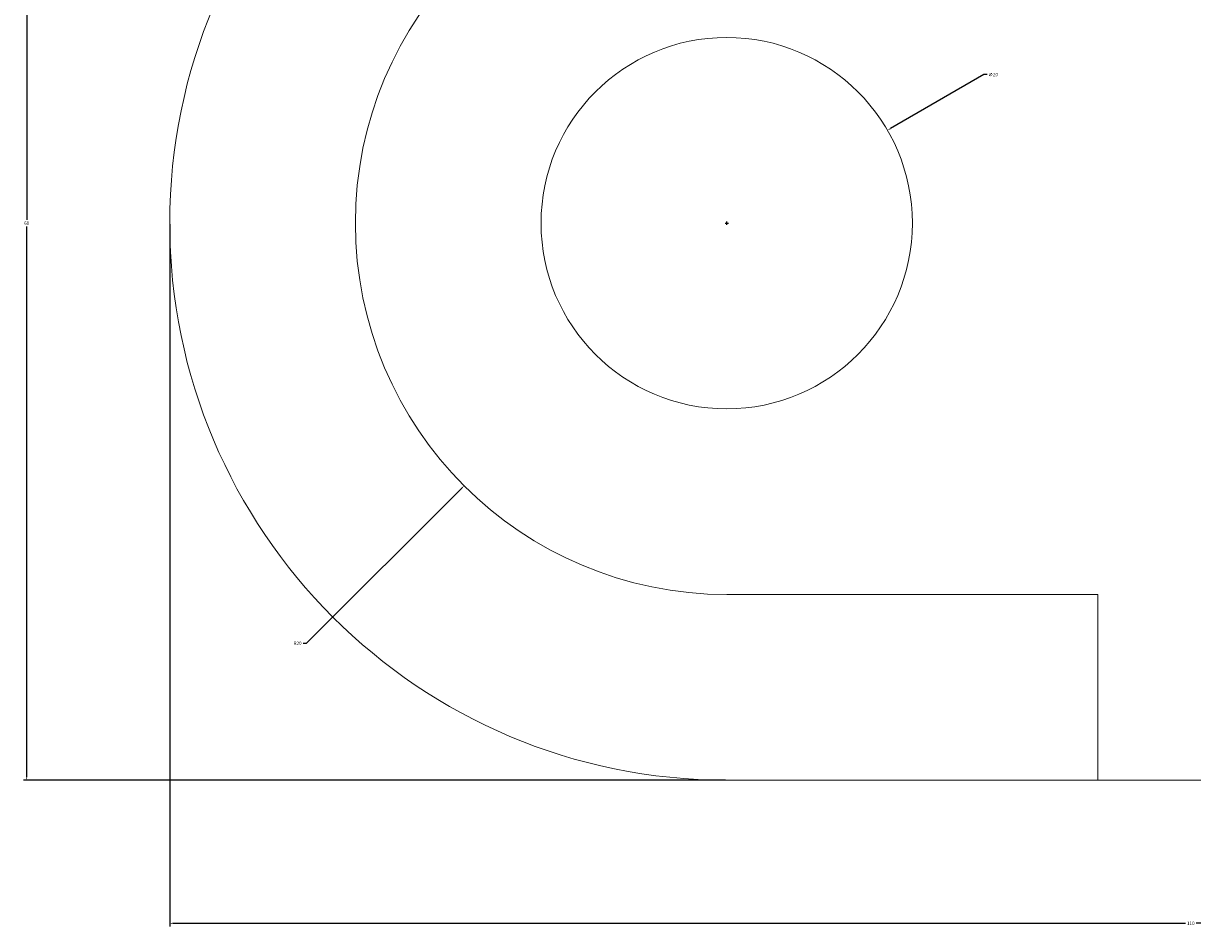
# Model space of a CAD drawing. Units: inches. Extents: x -19 to 107, y -27 to 49.
# Tile 1 of 4: x -19 to 44, y -27 to 22. Entities that reach past the tile are written whole.
import ezdxf

# ---------------------------------------------------------------- set-up
doc = ezdxf.new("R2010")
doc.units = ezdxf.units.IN
doc.header["$MEASUREMENT"] = 0
doc.layers.add('M-CONS', color=8, linetype='Continuous', lineweight=18)
doc.layers.add('M-DIMS', color=2, linetype='Continuous', lineweight=18)
doc.styles.get("Standard").update_dxf_attribs({"font": 'arial.ttf'})
doc.dimstyles.get("Standard").update_dxf_attribs({"dimtxt": 0.18, "dimasz": 0.18, "dimexe": 0.18, "dimexo": 0.0625, "dimgap": 0.09, "dimtad": 0, "dimtih": 1, "dimtoh": 1, "dimdec": 4, "dimzin": 0, "dimdsep": 46, "dimtxsty": 'Standard', "dimcen": 0.09, "dimadec": 0, "dimazin": 0, "dimtfac": 1, "dimtdec": 4, "dimtofl": 0, "dimtmove": 0, "dimatfit": 3, "dimfxl": 1, "dimtolj": 1, "dimtzin": 0, "dimarcsym": 0})

# ---------------------------------------------------------------- blocks, each defined once
blk = doc.blocks.new('*D1')
at = {"layer": 'Defpoints', "color": 0, "transparency": 16777216}
for p in [(-10.937, 10.82), (99.063, -19.18), (99.063, -26.885)]:
    blk.add_point(p, dxfattribs=at)
at = {"layer": 'M-DIMS', "color": 0, "lineweight": -2, "transparency": 16777216}
for p, q in [((-10.937, 10.758), (-10.937, -27.065)), ((99.063, -19.242), (99.063, -27.065)), ((-10.757, -26.885), (43.783, -26.885)), ((98.883, -26.885), (44.344, -26.885))]:
    blk.add_line(p, q, dxfattribs=at)
at = {"layer": 'M-DIMS', "color": 0, "transparency": 16777216}
for points in [[(-10.757, -26.855), (-10.757, -26.915), (-10.937, -26.885)], [(98.883, -26.855), (98.883, -26.915), (99.063, -26.885)]]:
    blk.add_solid(points, dxfattribs=at)
at = {"layer": 'M-DIMS', "color": 0, "transparency": 16777216, "insert": (44.063, -26.885), "char_height": 0.18, "attachment_point": 5}
blk.add_mtext('\\A1;110', dxfattribs=at)
blk = doc.blocks.new('*D2')
at = {"layer": 'Defpoints', "color": 0, "transparency": 16777216}
for p in [(-18.642, 40.82), (19.063, 40.82), (19.063, -19.18)]:
    blk.add_point(p, dxfattribs=at)
at = {"layer": 'M-DIMS', "color": 0, "lineweight": -2, "transparency": 16777216}
for p, q in [((19.001, 40.82), (-18.822, 40.82)), ((-18.642, 40.64), (-18.642, 11.002)), ((-18.642, -19), (-18.642, 10.638)), ((19.001, -19.18), (-18.822, -19.18))]:
    blk.add_line(p, q, dxfattribs=at)
at = {"layer": 'M-DIMS', "color": 0, "transparency": 16777216}
for points in [[(-18.672, 40.64), (-18.612, 40.64), (-18.642, 40.82)], [(-18.672, -19), (-18.612, -19), (-18.642, -19.18)]]:
    blk.add_solid(points, dxfattribs=at)
at = {"layer": 'M-DIMS', "color": 0, "transparency": 16777216, "insert": (-18.642, 10.82), "char_height": 0.18, "attachment_point": 5}
blk.add_mtext('\\A1;60', dxfattribs=at)
blk = doc.blocks.new('*D9')
at = {"layer": 'Defpoints', "color": 0, "transparency": 16777216}
for p in [(-2.151, 32.031), (19.063, 10.82)]:
    blk.add_point(p, dxfattribs=at)
at = {"layer": 'M-DIMS', "color": 0, "lineweight": -2, "transparency": 16777216}
for p, q in [((-15.06, 44.758), (-14.88, 44.758)), ((-14.88, 44.758), (-2.279, 32.159)), ((18.973, 10.82), (19.153, 10.82)), ((19.063, 10.73), (19.063, 10.91))]:
    blk.add_line(p, q, dxfattribs=at)
at = {"layer": 'M-DIMS', "color": 0, "transparency": 16777216}
blk.add_solid([(-2.258, 32.18), (-2.3, 32.138), (-2.151, 32.031)], dxfattribs=at)
at = {"layer": 'M-DIMS', "color": 0, "transparency": 16777216, "insert": (-15.365, 44.758), "char_height": 0.18, "attachment_point": 5}
blk.add_mtext('\\A1;R30', dxfattribs=at)
blk = doc.blocks.new('*D10')
at = {"layer": 'Defpoints', "color": 0, "transparency": 16777216}
for p in [(19.063, 10.82), (4.92, -3.32)]:
    blk.add_point(p, dxfattribs=at)
at = {"layer": 'M-DIMS', "color": 0, "lineweight": -2, "transparency": 16777216}
for p, q in [((18.973, 10.82), (19.153, 10.82)), ((19.063, 10.73), (19.063, 10.91)), ((-3.567, -11.805), (4.792, -3.448)), ((-3.747, -11.805), (-3.567, -11.805))]:
    blk.add_line(p, q, dxfattribs=at)
at = {"layer": 'M-DIMS', "color": 0, "transparency": 16777216}
blk.add_solid([(4.771, -3.426), (4.814, -3.469), (4.92, -3.32)], dxfattribs=at)
at = {"layer": 'M-DIMS', "color": 0, "transparency": 16777216, "insert": (-4.051, -11.805), "char_height": 0.18, "attachment_point": 5}
blk.add_mtext('\\A1;R20', dxfattribs=at)
blk = doc.blocks.new('*D11')
at = {"layer": 'Defpoints', "color": 0, "transparency": 16777216}
for p in [(27.724, 15.82), (10.403, 5.82)]:
    blk.add_point(p, dxfattribs=at)
at = {"layer": 'M-DIMS', "color": 0, "lineweight": -2, "transparency": 16777216}
for p, q in [((32.92, 18.82), (27.88, 15.91)), ((33.1, 18.82), (32.92, 18.82)), ((18.973, 10.82), (19.153, 10.82)), ((19.063, 10.73), (19.063, 10.91))]:
    blk.add_line(p, q, dxfattribs=at)
at = {"layer": 'M-DIMS', "color": 0, "transparency": 16777216}
blk.add_solid([(27.865, 15.936), (27.895, 15.884), (27.724, 15.82)], dxfattribs=at)
at = {"layer": 'M-DIMS', "color": 0, "transparency": 16777216, "insert": (33.417, 18.82), "char_height": 0.18, "attachment_point": 5}
blk.add_mtext('\\A1;∅20', dxfattribs=at)

msp = doc.modelspace()

# ---------------------------------------------------------------- linework, layer by layer
at = {"layer": 'M-CONS'}
for p, q in [((19.0635, -9.18, 20), (39.0635, -9.18, 20)), ((39.0635, -9.18, 20), (39.0635, -19.18, 20)), ((19.0635, -19.18), (99.0635, -19.18))]:
    msp.add_line(p, q, dxfattribs=at)
msp.add_circle((19.0635, 10.82, 20), 10, dxfattribs=at)
for centre, radius in [((19.0635, 10.82), 30), ((19.0635, 10.82, 20), 20)]:
    msp.add_arc(centre, radius, 90, 270, dxfattribs=at)

# ---------------------------------------------------------------- dimensions: what is measured, and where the dimension line sits
at = {"layer": 'M-DIMS'}
for mpoint, picture, middle in [((-2.1515, 32.0315), '*D9', (-15.3652, 44.7583)), ((4.9196, -3.3204), '*D10', (-4.0515, -11.8046))]:
    dim = msp.add_radius_dim(center=(19.0635, 10.82), mpoint=mpoint, dimstyle='Standard', override={"dimdec": 0, "dimlfac": 1, "dimrnd": 0, "dimzin": 0, "dimdsep": 46, "dimlunit": 2}, dxfattribs=at)
    dim.commit()
    dim.dimension.update_dxf_attribs({"geometry": picture, "text_midpoint": middle, "dimtype": 164})
dim = msp.add_linear_dim(base=(-18.6415, 40.82), p1=(19.0635, -19.18), p2=(19.0635, 40.82), angle=90, dimstyle='Standard', override={"dimdec": 0, "dimlfac": 1, "dimrnd": 0, "dimzin": 0, "dimdsep": 46, "dimlunit": 2}, dxfattribs=at)
dim.commit()
dim.dimension.update_dxf_attribs({"geometry": '*D2', "text_midpoint": (-18.6415, 10.82)})
dim = msp.add_diameter_dim_2p(p1=(10.4032, 5.8201), p2=(27.7238, 15.8199), dimstyle='Standard', override={"dimdec": 0, "dimlfac": 1, "dimrnd": 0, "dimzin": 0, "dimdsep": 46, "dimlunit": 2}, dxfattribs=at)
dim.commit()
dim.dimension.update_dxf_attribs({"geometry": '*D11', "text_midpoint": (33.4165, 18.8198), "dimtype": 163})
dim = msp.add_linear_dim(base=(99.0635, -26.885), p1=(-10.9365, 10.82), p2=(99.0635, -19.18), dimstyle='Standard', override={"dimdec": 0, "dimlfac": 1, "dimrnd": 0, "dimzin": 0, "dimdsep": 46, "dimlunit": 2}, dxfattribs=at)
dim.commit()
dim.dimension.update_dxf_attribs({"geometry": '*D1', "text_midpoint": (44.0635, -26.885)})

doc.saveas('drawing.dxf')
